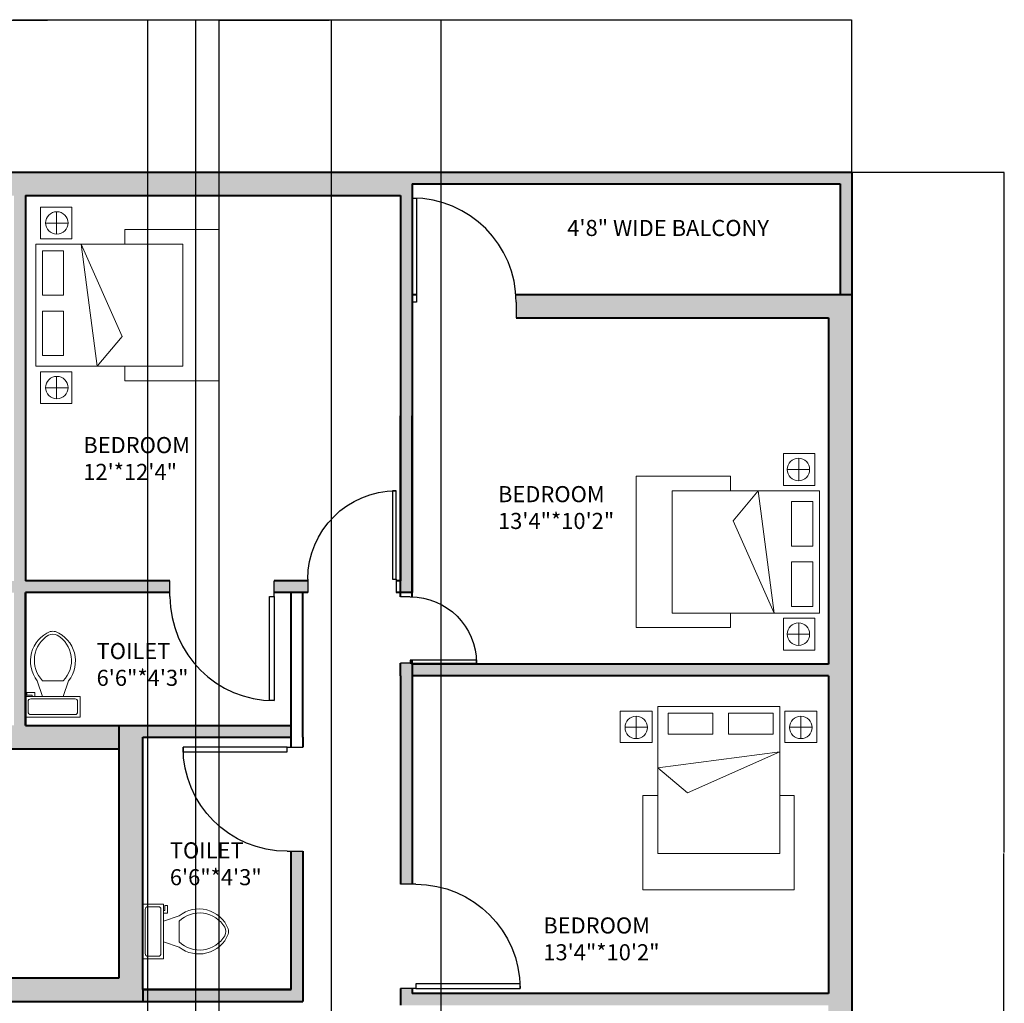
# Model space of a CAD drawing. Units: inches. Extents: x 1642 to 2399, y 1011 to 2291.
# Tile 7 of 7: x 2020 to 2399, y 1913 to 2291. Entities that reach past the tile are written whole.
import ezdxf

# ---------------------------------------------------------------- set-up
doc = ezdxf.new("R2010")
doc.units = ezdxf.units.IN
for name, color, linetype, lineweight in [('A-ANNO-DIMS', 2, 'Continuous', 18), ('A-AREA-IDEN', 7, 'Continuous', 20), ('A-DOOR', 4, 'Continuous', 25), ('A-FLOR-FIXT', 9, 'Continuous', 18), ('A-WALL-PATT', 40, 'Continuous', 13), ('BED', 200, 'Continuous', 18), ('WALL', 40, 'Continuous', 40)]:
    doc.layers.add(name, color=color, linetype=linetype, lineweight=lineweight)
doc.styles.get("Standard").update_dxf_attribs({"font": 'arial.ttf'})
doc.dimstyles.get("Standard").update_dxf_attribs({"dimtxt": 0.18, "dimasz": 0.18, "dimexe": 0.18, "dimexo": 0.0625, "dimgap": 0.09, "dimtad": 0, "dimtih": 1, "dimtoh": 1, "dimdec": 4, "dimzin": 0, "dimdsep": 46, "dimtxsty": 'Standard', "dimcen": 0.09, "dimadec": 0, "dimazin": 0, "dimtfac": 1, "dimtdec": 4, "dimtofl": 0, "dimtmove": 0, "dimatfit": 3, "dimfxl": 1, "dimtolj": 1, "dimtzin": 0, "dimarcsym": 0})

# ---------------------------------------------------------------- blocks, each defined once
blk = doc.blocks.new('*U2')
for p, q in [((0, 0), (0, -6)), ((40, 0), (40, -6))]:
    blk.add_line(p, q)
blk.add_lwpolyline([(0, 0), (0, 40), (1.75, 40), (1.75, 0)], close=True)
blk.add_arc((0, 0), 40, 0, 90)
blk = doc.blocks.new('*U4')
for p, q in [((9.5, -6), (9.5, -2)), ((-10, -8.5), (-8, -8.5)), ((-10, -9.5), (-10, -8.5)), ((-7, -9.5), (-10, -9.5)), ((-8, -8.5), (-8, -8)), ((-7, -8), (-7, -9.5)), ((-4, -8), (-6, -14)), ((4, -8), (6, -14)), ((4, -14), (-4, -14))]:
    blk.add_line(p, q)
blk.add_lwpolyline([(10.5, -8), (10.5, 0), (-10.5, 0), (-10.5, -8)], close=True)
for points in [[(-9.5, -2), (-9.5, -6)], [(8.5, -1), (-8.5, -1)], [(-8.5, -7), (8.5, -7)]]:
    blk.add_lwpolyline(points)
for centre, radius, start, end in [((-8.62, -1.88), 0.884, 81.8699, 188.1301), ((8.62, -1.88), 0.884, 351.8699, 98.1301), ((-8.62, -6.12), 0.884, 171.8699, 278.1301), ((8.62, -6.12), 0.884, 261.8699, 8.1301), ((3.52, -21.58), 12.17, 141.4691, 247.9714), ((4.2, -21.82), 11.33, 136.3677, 238.9468), ((-3.52, -21.58), 12.17, 292.0284, 38.5307), ((-4.2, -21.82), 11.33, 301.053, 43.6321), ((0, -27.88), 4, 245.7318, 294.2682), ((0, -29), 4, 254.8605, 285.1395)]:
    blk.add_arc(centre, radius, start, end)
blk = doc.blocks.new('BED-DOUBLE-WITH-NIGHTSTANDS')
for p, q in [((8.62, 34.13), (8.62, 70.38)), ((8.62, 70.38), (66.79, 70.38)), ((66.79, 70.38), (66.79, 34.13)), ((14.22, 34.13), (8.62, 34.13)), ((66.79, 34.13), (61.11, 34.13)), ((14.22, 17.36), (49.69, 33.17)), ((49.69, 33.17), (61.11, 23.59)), ((61.11, 23.59), (14.22, 17.36)), ((6.17, 3.76), (6.17, 12.35)), ((69.41, 3.76), (69.41, 12.35)), ((1.82, 7.94), (10.42, 7.94)), ((65.06, 7.94), (73.65, 7.94))]:
    blk.add_line(p, q)
for points in [[(14.22, 0), (61.11, 0), (61.11, 56.52), (14.22, 56.52)], [(12.24, 1.79), (0, 1.79), (0, 13.82), (12.24, 13.82)], [(75.48, 1.79), (63.24, 1.79), (63.24, 13.82), (75.48, 13.82)], [(16.77, 2.51), (33.87, 2.51), (33.87, 10.66), (16.77, 10.66)], [(39.94, 2.51), (57.04, 2.51), (57.04, 10.66), (39.94, 10.66)]]:
    blk.add_lwpolyline(points, close=True)
for centre in [(6.12, 8.05), (69.36, 8.05)]:
    blk.add_circle(centre, 4.3)
blk = doc.blocks.new('*D32')
at = {"layer": 'A-ANNO-DIMS', "color": 0, "lineweight": -2, "transparency": 16777216}
for p, q in [((1700.71, 2232.52), (1700.71, 2290.98)), ((1700.89, 2290.8), (2020.07, 2290.8)), ((2340.03, 2290.8), (2020.86, 2290.8)), ((2340.21, 2232.52), (2340.21, 2290.98))]:
    blk.add_line(p, q, dxfattribs=at)
at = {"layer": 'A-ANNO-DIMS', "color": 0, "transparency": 16777216}
for points in [[(1700.89, 2290.83), (1700.89, 2290.77), (1700.71, 2290.8)], [(2340.03, 2290.83), (2340.03, 2290.77), (2340.21, 2290.8)]]:
    blk.add_solid(points, dxfattribs=at)
at = {"layer": 'Defpoints', "color": 0, "transparency": 16777216}
for p in [(2340.21, 2290.8), (1700.71, 2232.46), (2340.21, 2232.46)]:
    blk.add_point(p, dxfattribs=at)
at = {"layer": 'A-ANNO-DIMS', "color": 0, "transparency": 16777216, "insert": (2020.46, 2290.8), "char_height": 0.18, "attachment_point": 5}
blk.add_mtext('\\A1;639.5', dxfattribs=at)
blk = doc.blocks.new('*D37')
at = {"layer": 'A-ANNO-DIMS', "color": 0, "lineweight": -2, "transparency": 16777216}
for p, q in [((2340.27, 2232.46), (2398.73, 2232.46)), ((2398.55, 2232.28), (2398.55, 1971.14)), ((2398.55, 1709.64), (2398.55, 1970.77)), ((2340.24, 1709.46), (2398.73, 1709.46))]:
    blk.add_line(p, q, dxfattribs=at)
at = {"layer": 'A-ANNO-DIMS', "color": 0, "transparency": 16777216}
for points in [[(2398.52, 2232.28), (2398.58, 2232.28), (2398.55, 2232.46)], [(2398.52, 1709.64), (2398.58, 1709.64), (2398.55, 1709.46)]]:
    blk.add_solid(points, dxfattribs=at)
at = {"layer": 'Defpoints', "color": 0, "transparency": 16777216}
for p in [(2340.21, 2232.46), (2398.55, 2232.46), (2340.18, 1709.46)]:
    blk.add_point(p, dxfattribs=at)
at = {"layer": 'A-ANNO-DIMS', "color": 0, "transparency": 16777216, "insert": (2398.55, 1970.96), "char_height": 0.18, "attachment_point": 5}
blk.add_mtext('\\A1;523', dxfattribs=at)
blk = doc.blocks.new('*D42')
at = {"layer": 'A-ANNO-DIMS', "color": 0, "lineweight": -2, "transparency": 16777216}
for p, q in [((1946.68, 1597.27), (1946.68, 2290.98)), ((1946.86, 2290.8), (2016.99, 2290.8)), ((2087.89, 2290.8), (2017.76, 2290.8)), ((2088.07, 1597.27), (2088.07, 2290.98))]:
    blk.add_line(p, q, dxfattribs=at)
at = {"layer": 'A-ANNO-DIMS', "color": 0, "transparency": 16777216}
for points in [[(1946.86, 2290.83), (1946.86, 2290.77), (1946.68, 2290.8)], [(2087.89, 2290.83), (2087.89, 2290.77), (2088.07, 2290.8)]]:
    blk.add_solid(points, dxfattribs=at)
at = {"layer": 'Defpoints', "color": 0, "transparency": 16777216}
for p in [(2088.07, 2290.8), (1946.68, 1597.21), (2088.07, 1597.21)]:
    blk.add_point(p, dxfattribs=at)
at = {"layer": 'A-ANNO-DIMS', "color": 0, "transparency": 16777216, "insert": (2017.37, 2290.8), "char_height": 0.18, "attachment_point": 5}
blk.add_mtext('\\A1;141.4', dxfattribs=at)
blk = doc.blocks.new('*D43')
at = {"layer": 'A-ANNO-DIMS', "color": 0, "lineweight": -2, "transparency": 16777216}
for p, q in [((2097.07, 1597.27), (2097.07, 2290.98)), ((2097.25, 2290.8), (2139.35, 2290.8)), ((2182.2, 2290.8), (2140.1, 2290.8)), ((2182.38, 1597.27), (2182.38, 2290.98))]:
    blk.add_line(p, q, dxfattribs=at)
at = {"layer": 'A-ANNO-DIMS', "color": 0, "transparency": 16777216}
for points in [[(2097.25, 2290.83), (2097.25, 2290.77), (2097.07, 2290.8)], [(2182.2, 2290.83), (2182.2, 2290.77), (2182.38, 2290.8)]]:
    blk.add_solid(points, dxfattribs=at)
at = {"layer": 'Defpoints', "color": 0, "transparency": 16777216}
for p in [(2182.38, 2290.8), (2097.07, 1597.21), (2182.38, 1597.21)]:
    blk.add_point(p, dxfattribs=at)
at = {"layer": 'A-ANNO-DIMS', "color": 0, "transparency": 16777216, "insert": (2139.72, 2290.8), "char_height": 0.18, "attachment_point": 5}
blk.add_mtext('\\A1;85.31', dxfattribs=at)
blk = doc.blocks.new('*D48')
at = {"layer": 'A-ANNO-DIMS', "color": 0, "lineweight": -2, "transparency": 16777216}
for p, q in [((1922.74, 1392.77), (1922.74, 2290.98)), ((1922.92, 2290.8), (2031.1, 2290.8)), ((2140.06, 2290.8), (2031.89, 2290.8)), ((2140.24, 1392.77), (2140.24, 2290.98))]:
    blk.add_line(p, q, dxfattribs=at)
at = {"layer": 'A-ANNO-DIMS', "color": 0, "transparency": 16777216}
for points in [[(1922.92, 2290.83), (1922.92, 2290.77), (1922.74, 2290.8)], [(2140.06, 2290.83), (2140.06, 2290.77), (2140.24, 2290.8)]]:
    blk.add_solid(points, dxfattribs=at)
at = {"layer": 'Defpoints', "color": 0, "transparency": 16777216}
for p in [(2140.24, 2290.8), (1922.74, 1392.71), (2140.24, 1392.71)]:
    blk.add_point(p, dxfattribs=at)
at = {"layer": 'A-ANNO-DIMS', "color": 0, "transparency": 16777216, "insert": (2031.49, 2290.8), "char_height": 0.18, "attachment_point": 5}
blk.add_mtext('\\A1;217.5', dxfattribs=at)
blk = doc.blocks.new('*D50')
at = {"layer": 'A-ANNO-DIMS', "color": 0, "lineweight": -2, "transparency": 16777216}
for p, q in [((1993.24, 1295.77), (1993.24, 2290.98)), ((1993.42, 2290.8), (2031.17, 2290.8)), ((2069.56, 2290.8), (2031.82, 2290.8)), ((2069.74, 1295.77), (2069.74, 2290.98))]:
    blk.add_line(p, q, dxfattribs=at)
at = {"layer": 'A-ANNO-DIMS', "color": 0, "transparency": 16777216}
for points in [[(1993.42, 2290.83), (1993.42, 2290.77), (1993.24, 2290.8)], [(2069.56, 2290.83), (2069.56, 2290.77), (2069.74, 2290.8)]]:
    blk.add_solid(points, dxfattribs=at)
at = {"layer": 'Defpoints', "color": 0, "transparency": 16777216}
for p in [(2069.74, 2290.8), (1993.24, 1295.71), (2069.74, 1295.71)]:
    blk.add_point(p, dxfattribs=at)
at = {"layer": 'A-ANNO-DIMS', "color": 0, "transparency": 16777216, "insert": (2031.49, 2290.8), "char_height": 0.18, "attachment_point": 5}
blk.add_mtext('\\A1;76.5', dxfattribs=at)

msp = doc.modelspace()

# ---------------------------------------------------------------- hatches: boundary and pattern name
at = {"layer": 'A-WALL-PATT'}
h = msp.add_hatch(color=256, dxfattribs=at)
h.dxf.hatch_style = 1
h.paths.add_polyline_path([(2340.1804, 2185.4562), (2211.0983, 2185.4562, -0.01876983), (2211.211, 2182.4562), (2211.211, 2176.4562), (2331.211, 2176.4562), (2331.211, 2043.4562), (2171.211, 2043.4562), (2171.211, 2038.9562), (2331.211, 2038.9562), (2331.211, 1916.9562), (2171.211, 1916.9562), (2171.211, 1918.9365), (2166.711, 1918.9365), (2166.711, 1912.4562), (2340.1804, 1912.4562)])
h.paths.add_polyline_path([(2171.211, 2043.4562), (2171.211, 2043.9025), (2170.5217, 2043.9025), (2166.711, 2043.9025), (2166.711, 2038.9562), (2166.711, 1958.9365), (2171.211, 1958.9365)], flags=17)
h.paths.add_polyline_path([(2129.211, 1971.5979), (2124.711, 1971.5979), (2124.711, 1918.4562), (2067.711, 1918.4562), (2067.711, 1913.9562), (2129.211, 1913.9562)])
h.paths.add_polyline_path([(2067.711, 2015.4562), (2124.711, 2015.4562), (2124.711, 2019.9562), (2058.711, 2019.9562), (2058.711, 2015.4562), (2058.711, 1922.9562), (1982.211, 1922.9562), (1982.211, 2015.4562), (1982.211, 2019.9562), (1916.211, 2019.9562), (1916.211, 2070.9562), (1911.711, 2070.9562), (1911.711, 2015.4562), (1911.711, 2012.302), (1916.211, 2012.302), (1916.211, 2015.4562), (1973.211, 2015.4562), (1973.211, 1918.4562), (1973.211, 1913.9562), (2017.1804, 1913.9562), (2067.711, 1913.9562), (2067.711, 1918.4562)])
h.paths.add_polyline_path([(2131.1386, 2075.4562), (2118.1934, 2075.4562), (2118.1934, 2070.9562), (2131.1386, 2070.9562)], flags=17)
h.paths.add_polyline_path([(1918.8034, 2075.4562), (1909.4956, 2075.4562), (1909.4956, 2070.9562), (1918.8034, 2070.9562)], flags=17)
h.paths.add_polyline_path([(1874.211, 2029.9562), (1869.711, 2029.9562), (1869.711, 1960.7404), (1874.211, 1960.7404)], flags=17)
h.paths.add_polyline_path([(1916.211, 1972.302), (1911.711, 1972.302), (1911.711, 1918.4562), (1916.211, 1918.4562)], flags=17)
h.paths.add_polyline_path([(2340.1804, 1912.4562), (2331.1804, 1912.4562), (2331.1804, 1794.4562), (2210.1804, 1794.4562), (2210.1804, 1789.9562), (2279.6804, 1789.9562), (2340.1804, 1789.9562)])
h.paths.add_polyline_path([(2288.6804, 1789.9562), (2279.6804, 1789.9562), (2279.6804, 1785.0846), (2285.6804, 1785.0846), (2288.6804, 1785.0846)], flags=17)
h.paths.add_polyline_path([(2169.6804, 1789.9562), (2170.1804, 1789.9562), (2170.1804, 1794.4562), (2165.1804, 1794.4562), (2165.1804, 1713.9562), (2165.1804, 1709.4562), (2279.6804, 1709.4562), (2279.6804, 1718.4562), (2169.6804, 1718.4562)])
h.paths.add_polyline_path([(2288.6804, 1745.1973, -0.01876983), (2285.6804, 1745.0846), (2279.6804, 1745.0846), (2279.6804, 1709.4562), (2340.1804, 1709.4562), (2340.1804, 1789.9562), (2335.6804, 1789.9562), (2335.6804, 1713.9562), (2288.6804, 1713.9562)])
h.paths.add_polyline_path([(2165.1804, 1713.9562), (2140.6229, 1713.9562), (2088.923, 1713.9562), (2069.7509, 1713.9562), (2060.4457, 1713.9562), (2060.4457, 1709.4562), (2165.1804, 1709.4562)])
h.paths.add_polyline_path([(2020.4457, 1713.9562), (2017.1804, 1713.9562), (2012.6804, 1713.9562), (2009.1946, 1713.9562), (2009.1946, 1709.4562), (2020.4457, 1709.4562)])
h.paths.add_polyline_path([(1969.1946, 1713.9562), (1864.6804, 1713.9562), (1864.6804, 1798.9562), (1860.1804, 1798.9562), (1860.1804, 1792.9562), (1860.1804, 1752.9562), (1860.1804, 1718.4562), (1750.1804, 1718.4562), (1750.1804, 1749.2419), (1744.1804, 1749.2419, -0.01876983), (1741.1804, 1749.3546), (1741.1804, 1709.4562), (1969.1946, 1709.4562)])
h.paths.add_polyline_path([(1741.1804, 1803.4562), (1700.711, 1803.4562), (1700.711, 1794.4562), (1741.1804, 1794.4562)])
h.paths.add_polyline_path([(1820.1804, 1798.9562), (1741.1804, 1798.9562), (1741.1804, 1794.4562), (1741.1804, 1790.0365), (1741.1804, 1789.2419), (1744.1804, 1789.2419), (1750.1804, 1789.2419), (1750.1804, 1794.4562), (1820.1804, 1794.4562)], flags=17)
h.paths.add_polyline_path([(1800.6804, 1709.4562), (1796.1804, 1709.4562), (1796.1804, 1592.7078), (1978.9325, 1592.7078), (1978.9325, 1597.2078), (1800.6804, 1597.2078)])
h.paths.add_polyline_path([(2097.0678, 1709.4562), (2088.0678, 1709.4562), (2088.0678, 1599.6874), (2088.0678, 1597.2078), (2097.0678, 1597.2078)], flags=17)
h.paths.add_polyline_path([(2186.8766, 1709.4562), (2182.3766, 1709.4562), (2182.3766, 1597.2078), (2071.4624, 1597.2078), (2071.4624, 1592.7078), (2186.8766, 1592.7078)])
h.paths.add_polyline_path([(2078.1934, 2075.4562), (2022.711, 2075.4562), (2022.711, 2223.4562), (2166.711, 2223.4562), (2166.711, 2075.4562), (2166.711, 2070.9562), (2171.211, 2070.9562), (2171.211, 2138.8919), (2171.211, 2227.9562), (2335.711, 2227.9562), (2335.711, 2185.4562), (2340.1804, 2185.4562), (2340.1804, 2232.4562), (1874.211, 2232.4562), (1874.211, 2223.4562), (2018.211, 2223.4562), (2018.211, 2075.4562), (1958.8034, 2075.4562), (1958.8034, 2070.9562), (2018.211, 2070.9562), (2018.211, 2019.9562), (1982.211, 2019.9562), (1982.211, 2015.4562), (1982.211, 2010.9562), (2058.711, 2010.9562), (2058.711, 2015.4562), (2058.711, 2019.9562), (2022.711, 2019.9562), (2022.711, 2070.9562), (2078.1934, 2070.9562)])
h.paths.add_polyline_path([(1874.211, 2171.9562), (1874.211, 2176.4562), (1861.9371, 2176.4562), (1861.9371, 2173.4562), (1861.9371, 2167.4562), (1869.711, 2167.4562), (1869.711, 2069.7602), (1874.211, 2069.7602)], flags=17)
h.paths.add_polyline_path([(1705.211, 2227.9562), (1865.211, 2227.9562), (1865.211, 2176.4562), (1874.211, 2176.4562), (1874.211, 2232.4562), (1700.711, 2232.4562), (1700.711, 2176.4562), (1705.211, 2176.4562)])
h.paths.add_polyline_path([(1709.711, 2167.4562), (1821.9371, 2167.4562), (1821.9371, 2173.4562, -0.01876983), (1822.0498, 2176.4562), (1700.711, 2176.4562), (1700.711, 1913.9562), (1860.1804, 1913.9562), (1864.6804, 1913.9562), (1973.211, 1913.9562), (1973.211, 1918.4562), (1916.211, 1918.4562), (1874.211, 1918.4562), (1874.211, 1920.7404), (1869.711, 1920.7404), (1869.711, 1918.4562), (1860.1804, 1918.4562), (1709.711, 1918.4562), (1709.711, 2029.9562), (1874.211, 2029.9562), (1874.211, 2037.0364), (1869.711, 2037.0364), (1869.711, 2034.4562), (1709.711, 2034.4562)])
h.paths.add_polyline_path([(2017.1804, 1913.9562), (2012.6804, 1913.9562), (2012.6804, 1713.9562), (2017.1804, 1713.9562)])
h.paths.add_polyline_path([(1952.4341, 2110.3716), (2000.4134, 2110.3716), (2000.4134, 2133.4189), (1952.4341, 2133.4189)], flags=25)
h.paths.add_polyline_path([(2042.3983, 2110.7121), (2090.3775, 2110.7121), (2090.3775, 2133.7594), (2042.3983, 2133.7594)], flags=25)
h.paths.add_polyline_path([(2201.7332, 2091.8715), (2249.7125, 2091.8715), (2249.7125, 2114.9188), (2201.7332, 2114.9188)], flags=25)
h.paths.add_polyline_path([(1805.186, 2077.6915), (1853.1653, 2077.6915), (1853.1653, 2100.7388), (1805.186, 2100.7388)], flags=25)
h.paths.add_polyline_path([(1794.8897, 1974.6584), (1842.869, 1974.6584), (1842.869, 1997.7057), (1794.8897, 1997.7057)], flags=25)
h.paths.add_polyline_path([(2229.1796, 2204.4209), (2315.1362, 2204.4209), (2315.1362, 2217.1488), (2229.1796, 2217.1488)], flags=25)
h.paths.add_polyline_path([(1715.2159, 2199.5328), (1801.1724, 2199.5328), (1801.1724, 2212.2607), (1715.2159, 2212.2607)], flags=25)
h.paths.add_polyline_path([(2230.7681, 1755.7109), (2271.7283, 1755.7109), (2271.7283, 1778.7582), (2230.7681, 1778.7582)], flags=25)
h.paths.add_polyline_path([(1763.4713, 1764.1742), (1804.4315, 1764.1742), (1804.4315, 1787.2215), (1763.4713, 1787.2215)], flags=25)
h.paths.add_polyline_path([(2076.2643, 1955.0495), (2111.326, 1955.0495), (2111.326, 1978.0968), (2076.2643, 1978.0968)], flags=25)
h.paths.add_polyline_path([(1932.854, 1956.1217), (1967.9158, 1956.1217), (1967.9158, 1979.169), (1932.854, 1979.169)], flags=25)
h.paths.add_polyline_path([(2048.1203, 2031.6107), (2083.1821, 2031.6107), (2083.1821, 2054.658), (2048.1203, 2054.658)], flags=25)
h.paths.add_polyline_path([(2163.5754, 1863.7569), (2208.2347, 1863.7569), (2208.2347, 1886.8042), (2163.5754, 1886.8042)], flags=9)
h.paths.add_polyline_path([(2039.9286, 1809.0957), (2084.5879, 1809.0957), (2084.5879, 1832.143), (2039.9286, 1832.143)], flags=9)
h.paths.add_polyline_path([(1901.0045, 1814.0452), (1945.6638, 1814.0452), (1945.6638, 1837.0925), (1901.0045, 1837.0925)], flags=9)
h.paths.add_polyline_path([(1833.7282, 1852.5627), (1878.3875, 1852.5627), (1878.3875, 1875.61), (1833.7282, 1875.61)], flags=9)
h.paths.add_polyline_path([(2219.1375, 1926.2139), (2267.1167, 1926.2139), (2267.1167, 1949.2612), (2219.1375, 1949.2612)], flags=25)
h.paths.add_polyline_path([(1956.9598, 2029.7735), (1992.0216, 2029.7735), (1992.0216, 2052.8208), (1956.9598, 2052.8208)], flags=25)
h.paths.add_polyline_path([(2229.3, 1523.3399), (2270.2602, 1523.3399), (2270.2602, 1546.3872), (2229.3, 1546.3872)], flags=9)
h.paths.add_polyline_path([(1772.3039, 1526.9922), (1813.2641, 1526.9922), (1813.2641, 1550.0394), (1772.3039, 1550.0394)], flags=9)
h.paths.add_polyline_path([(2172.587, 1420.6999), (2217.2463, 1420.6999), (2217.2463, 1443.7472), (2172.587, 1443.7472)], flags=9)
h.paths.add_polyline_path([(1814.3549, 1422.215), (1859.0143, 1422.215), (1859.0143, 1445.2623), (1814.3549, 1445.2623)], flags=9)
h.paths.add_polyline_path([(2186.0372, 1305.6227), (2234.0165, 1305.6227), (2234.0165, 1328.67), (2186.0372, 1328.67)], flags=9)
h.paths.add_polyline_path([(1756.747, 1349.0694), (1804.7263, 1349.0694), (1804.7263, 1372.1167), (1756.747, 1372.1167)], flags=9)
h.paths.add_polyline_path([(2239.449, 1214.6184), (2287.4282, 1214.6184), (2287.4282, 1237.6657), (2239.449, 1237.6657)], flags=9)
h.paths.add_polyline_path([(1767.104, 1213.8348), (1815.0832, 1213.8348), (1815.0832, 1236.8821), (1767.104, 1236.8821)], flags=9)
h.paths.add_polyline_path([(2046.6809, 1183.6854), (2094.6602, 1183.6854), (2094.6602, 1206.7327), (2046.6809, 1206.7327)], flags=9)
h.paths.add_polyline_path([(1947.2155, 1183.6854), (1995.1948, 1183.6854), (1995.1948, 1206.7327), (1947.2155, 1206.7327)], flags=9)
h.paths.add_polyline_path([(1959.3556, 1258.7871), (1994.4174, 1258.7871), (1994.4174, 1281.8344), (1959.3556, 1281.8344)], flags=9)
h.paths.add_polyline_path([(2049.6419, 1248.9629), (2084.7036, 1248.9629), (2084.7036, 1272.0102), (2049.6419, 1272.0102)], flags=9)
h.paths.add_polyline_path([(2092.7532, 1327.4852), (2127.815, 1327.4852), (2127.815, 1350.5325), (2092.7532, 1350.5325)], flags=9)
h.paths.add_polyline_path([(1944.9358, 1327.4852), (1979.9976, 1327.4852), (1979.9976, 1350.5325), (1944.9358, 1350.5325)], flags=9)
h.paths.add_polyline_path([(1974.5055, 1650.063), (2006.3695, 1650.063), (2006.3695, 1662.7909), (1974.5055, 1662.7909)], flags=9)

# ---------------------------------------------------------------- linework, layer by layer
at = {"layer": 'WALL'}
for p, q in [((1874.211, 2232.4562), (2022.711, 2232.4562)), ((2022.711, 2232.4562), (2171.211, 2232.4562)), ((2171.211, 2232.4562), (2340.211, 2232.4562)), ((2340.211, 2232.4562), (2340.211, 2178.162)), ((2171.211, 2227.9562), (2171.211, 2070.9562)), ((2171.211, 2227.9562), (2335.711, 2227.9562)), ((2335.711, 2227.9562), (2335.711, 2185.4562)), ((2022.711, 2223.4562), (2022.711, 2075.4562)), ((2022.711, 2223.4562), (2166.711, 2223.4562)), ((2166.711, 2223.4562), (2166.711, 2075.4562)), ((2171.211, 2185.4562), (2172.961, 2185.4562)), ((2211.0983, 2185.4562), (2340.211, 2185.4562)), ((2340.211, 2185.4562), (2340.211, 2038.9562)), ((2211.211, 2176.4562), (2223.211, 2176.4562)), ((2211.211, 2176.4562), (2331.211, 2176.4562)), ((2331.211, 2176.4562), (2331.211, 2043.4562)), ((2166.711, 2069.3076), (2166.711, 2138.8919)), ((2171.211, 2069.2983), (2171.211, 2138.8919)), ((2078.1934, 2075.4562), (2022.711, 2075.4562)), ((2131.1386, 2075.4562), (2118.1934, 2075.4562)), ((2166.711, 2075.4562), (2165.1458, 2075.4562)), ((2022.711, 2070.9562), (2022.711, 2019.9562)), ((2022.711, 2019.9562), (2022.711, 2070.9562)), ((2078.1934, 2070.9562), (2022.711, 2070.9562)), ((2131.1386, 2070.9562), (2118.1934, 2070.9562)), ((2124.711, 2019.9562), (2124.711, 2070.9562)), ((2129.211, 2015.4562), (2129.211, 2070.9562)), ((2171.211, 2070.9562), (2165.1458, 2070.9562)), ((2166.711, 2038.9562), (2166.711, 2043.9025)), ((2171.211, 2043.4562), (2171.211, 2045.014)), ((2331.211, 2043.4562), (2171.211, 2043.4562)), ((2171.211, 2043.4562), (2171.211, 1958.9365)), ((2124.711, 2011.5979), (2124.711, 2037.5317)), ((2166.711, 2038.9562), (2166.711, 1958.9365)), ((2331.211, 2038.9562), (2171.211, 2038.9562)), ((2331.211, 2038.9562), (2331.211, 1916.9562)), ((2340.211, 2038.9562), (2340.211, 1912.4562)), ((2022.711, 2019.9562), (2124.711, 2019.9562)), ((2058.711, 2015.4562), (2058.711, 2019.9562)), ((2058.711, 1922.9562), (2058.711, 2015.4562)), ((2067.711, 2015.4562), (2124.711, 2015.4562)), ((2067.711, 1918.4562), (2067.711, 2015.4562)), ((2129.211, 2015.4562), (2129.211, 2011.5979)), ((1982.211, 2010.9562), (2058.711, 2010.9562)), ((2124.711, 1918.4562), (2124.711, 1971.5979)), ((2129.211, 1971.5979), (2129.211, 1913.9562)), ((1982.211, 1922.9562), (2058.711, 1922.9562)), ((2067.711, 1918.4562), (2124.711, 1918.4562)), ((2124.711, 1918.4562), (2067.711, 1918.4562)), ((2067.711, 1918.4562), (2067.711, 1913.9562)), ((2166.711, 1918.9365), (2166.711, 1912.4562)), ((2171.211, 1918.9365), (2171.211, 1916.9562)), ((2331.211, 1916.9562), (2171.211, 1916.9562)), ((2012.6804, 1913.9562), (2129.211, 1913.9562))]:
    msp.add_line(p, q, dxfattribs=at)
msp.add_lwpolyline([(1969.1946, 1709.4562), (1700.711, 1709.4562), (1700.711, 2232.4562), (2340.1804, 2232.4562), (2340.1804, 1709.4562), (2060.4457, 1709.4562)], dxfattribs=at)

# ---------------------------------------------------------------- block references
at = {"layer": 'A-DOOR'}
msp.add_blockref('*U2', (2171.211, 2182.4562), dxfattribs=at)
at = {"layer": 'A-DOOR', "xscale": -0.8501804344082186, "yscale": 0.8501804344082186, "zscale": 0.8501804344082186}
msp.add_blockref('*U2', (2165.1458, 2076.0573), dxfattribs=at)
at = {"layer": 'A-DOOR', "rotation": 180}
msp.add_blockref('*U2', (2118.1934, 2069.4562), dxfattribs=at)
at = {"layer": 'A-DOOR', "xscale": -0.6351273996805391, "yscale": 0.6351273996805391, "zscale": 0.6351273996805391, "rotation": 270}
msp.add_blockref('*U2', (2170.5217, 2043.9025), dxfattribs=at)
at = {"layer": 'A-DOOR', "xscale": -1}
for p, rotation in [((2123.211, 2011.5979), 90), ((2172.711, 1918.9365), 270)]:
    msp.add_blockref('*U2', p, dxfattribs=dict(at, rotation=rotation))
at = {"layer": 'A-FLOR-FIXT', "xscale": -1}
for p, rotation in [((2033.211, 2023.1011), 180), ((2067.711, 1940.7894), 90)]:
    msp.add_blockref('*U4', p, dxfattribs=dict(at, rotation=rotation))
at = {"layer": 'BED'}
for p, rotation in [((2026.6711, 2219.0326), 270.0000000000004), ((2327.7133, 2048.8687), 90.00000000000072), ((2326.6883, 2027.2023), 180)]:
    msp.add_blockref('BED-DOUBLE-WITH-NIGHTSTANDS', p, dxfattribs=dict(at, rotation=rotation))

# ---------------------------------------------------------------- texts
at = {"layer": 'A-AREA-IDEN', "attachment_point": 1}
for s, insert, char_height in [('4\'8" WIDE BALCONY', (2230.8333, 2214.0795), 6.176468), ('BEDROOM\\P12\'*12\'4"', (2044.8819, 2130.6901), 6.17647), ('BEDROOM\\P13\'4"*10\'2"', (2204.2169, 2111.8496), 6.176468), ('TOILET\\P6\'6"*4\'3"', (2049.9888, 2051.5887), 6.17647), ('TOILET\\P6\'6"*4\'3"', (2078.1328, 1975.0275), 6.17647), ('BEDROOM\\P13\'4"*10\'2"', (2221.6211, 1946.1919), 6.176468)]:
    msp.add_mtext_dynamic_manual_height_columns(s, width=136.850471, gutter_width=30.8823, heights=[0], dxfattribs=dict(at, insert=insert, char_height=char_height))

# ---------------------------------------------------------------- dimensions: what is measured, and where the dimension line sits
at = {"layer": 'A-ANNO-DIMS'}
for base, p1, p2, override, picture, middle in [((2340.211, 2290.7962), (1700.711, 2232.4562), (2340.211, 2232.4562), {"dimdec": 1, "dimlfac": 1, "dimrnd": 0, "dimzin": 0, "dimdsep": 46, "dimlunit": 2}, '*D32', (2020.461, 2290.7962)), ((2140.2415, 2290.7962), (1922.7415, 1392.7078), (2140.2415, 1392.7078), {"dimdec": 1, "dimlfac": 1, "dimrnd": 0, "dimzin": 0, "dimdsep": 46, "dimlunit": 2}, '*D48', (2031.4915, 2290.7962)), ((2088.0678, 2290.7962), (1946.6804, 1597.2078), (2088.0678, 1597.2078), {"dimdec": 1, "dimlfac": 1, "dimrnd": 0, "dimzin": 0, "dimdsep": 46, "dimlunit": 2}, '*D42', (2017.3741, 2290.7962)), ((2069.7415, 2290.7962), (1993.2415, 1295.7078), (2069.7415, 1295.7078), {"dimdec": 1, "dimlfac": 1, "dimrnd": 0, "dimzin": 0, "dimdsep": 46, "dimlunit": 2}, '*D50', (2031.4915, 2290.7962)), ((2182.3766, 2290.7962), (2097.0678, 1597.2078), (2182.3766, 1597.2078), {"dimdec": 2, "dimlfac": 1, "dimrnd": 0, "dimzin": 0, "dimdsep": 46, "dimlunit": 2}, '*D43', (2139.7222, 2290.7962))]:
    dim = msp.add_linear_dim(base=base, p1=p1, p2=p2, dimstyle='Standard', override=override, dxfattribs=at)
    dim.commit()
    dim.dimension.update_dxf_attribs({"geometry": picture, "text_midpoint": middle})
dim = msp.add_linear_dim(base=(2398.551, 2232.4562), p1=(2340.1804, 1709.4562), p2=(2340.211, 2232.4562), angle=90, dimstyle='Standard', override={"dimdec": 0, "dimlfac": 1, "dimrnd": 0, "dimzin": 0, "dimdsep": 46, "dimlunit": 2}, dxfattribs=at)
dim.commit()
dim.dimension.update_dxf_attribs({"geometry": '*D37', "text_midpoint": (2398.551, 1970.9562)})

doc.saveas('drawing.dxf')
